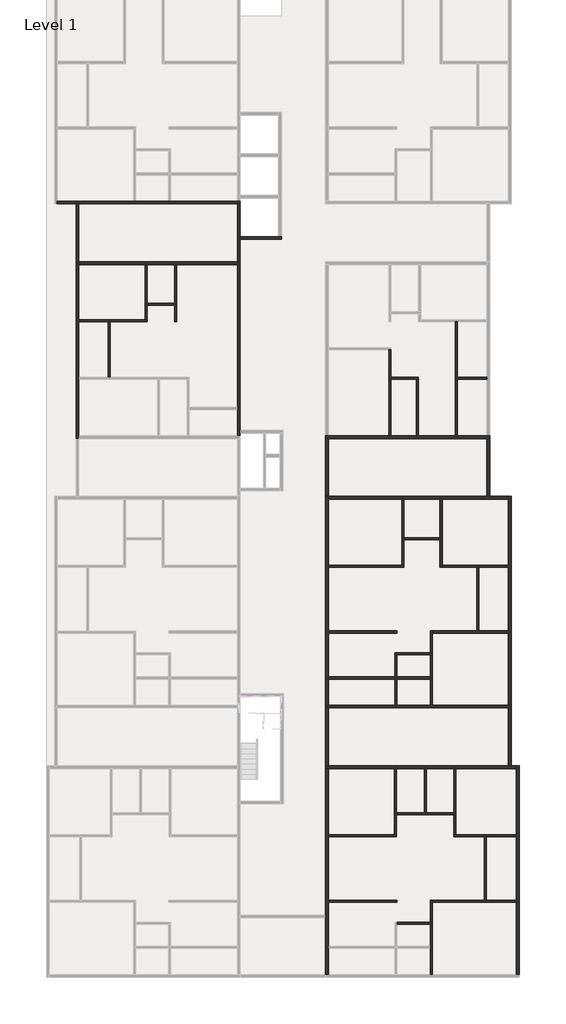
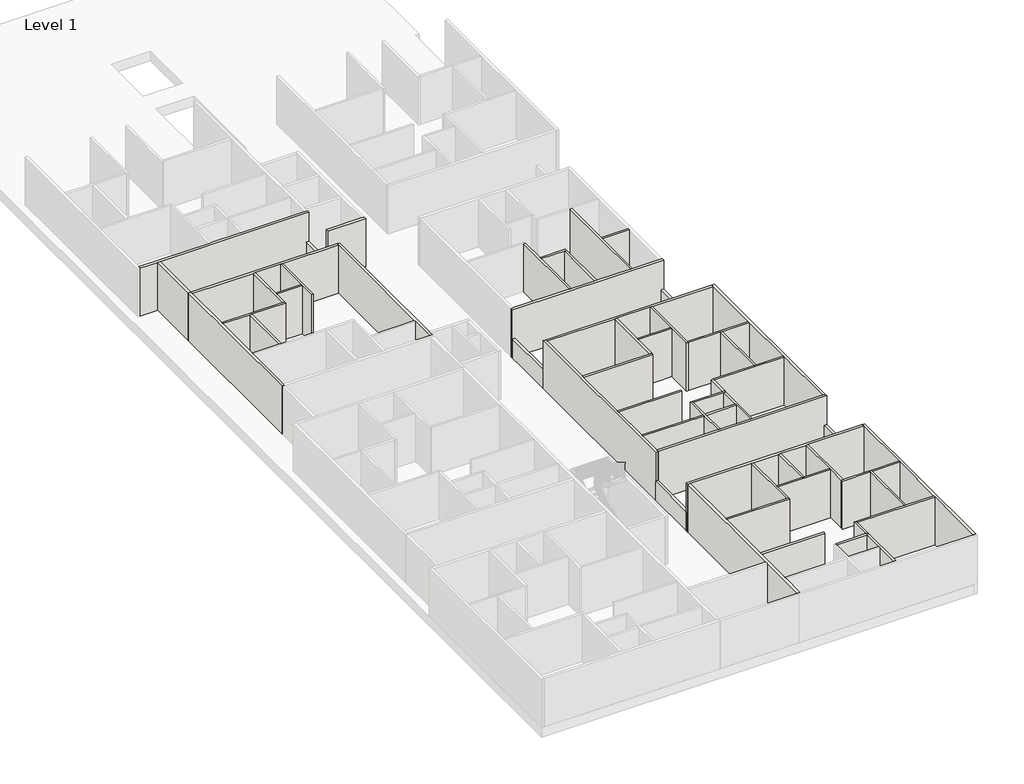
# One storey, part 2 of 8: 56 walls.
"""IFC4 building model written with IfcOpenShell, lengths in millimetres."""

from ifc_helpers import new_model, si_unit, frame, origin, place, context, project, spatial, polyline, outline, extrude, faceted_brep, element, save

model = new_model("IFC4")

# Units and contexts
model_context = context("Model", 3, world=origin())
ifc_project = project(units=[si_unit("LENGTHUNIT", "METRE", prefix="MILLI")], contexts=[model_context])

# Site, building, storey
site = spatial("IfcSite", under=ifc_project)
building = spatial("IfcBuilding", under=site)
storey = spatial("IfcBuildingStorey", under=building, Name="Level 1", Elevation=25234.6172466)

# Walls
placement = place(None, origin())
element("IfcWall", 1, ObjectType="4.5\"", at=placement, inside=storey, context=model_context, shape_type="Brep", body=[
    faceted_brep([(-12531.5544854, 2100.0216096, 25234.6172466), (-10907.2415084, 2100.0216096, 25234.6172466), (-10792.9415084, 2100.0216096, 25234.6172466), (-8759.6544854, 2100.0216096, 25234.6172466), (-8759.6544854, 2100.0216096, 28282.6172466), (-10792.9415084, 2100.0216096, 28282.6172466), (-10907.2415084, 2100.0216096, 28282.6172466), (-12531.5544854, 2100.0216096, 28282.6172466), (-12531.5544854, 2214.3216096, 25234.6172466), (-12531.5544854, 2214.3216096, 28282.6172466), (-8873.9544854, 2214.3216096, 28282.6172466), (-8759.6544854, 2214.3216096, 28282.6172466), (-8759.6544854, 2214.3216096, 25234.6172466), (-8873.9544854, 2214.3216096, 25234.6172466)], [[[0, 1, 2, 3, 4, 5, 6, 7]], [[8, 9, 10, 11, 12, 13]], [[3, 2, 1, 0, 8, 13, 12]], [[0, 7, 9, 8]], [[4, 3, 12, 11]], [[7, 6, 5, 4, 11, 10, 9]]]),
])
element("IfcWall", 2, ObjectType="4.5\"", at=placement, inside=storey, context=model_context, shape_type="Brep", body=[
    faceted_brep([(-8759.6544854, 2214.3216096, 25234.6172466), (-8759.6544854, 3014.4216096, 25234.6172466), (-8759.6544854, 3128.7216096, 25234.6172466), (-8759.6544854, 5264.2743917, 25234.6172466), (-8759.6544854, 5264.2743917, 28282.6172466), (-8759.6544854, 3128.7216096, 28282.6172466), (-8759.6544854, 3014.4216096, 28282.6172466), (-8759.6544854, 2214.3216096, 28282.6172466), (-8873.9544854, 2214.3216096, 25234.6172466), (-8873.9544854, 2214.3216096, 28282.6172466), (-8873.9544854, 5264.2743917, 28282.6172466), (-8873.9544854, 5264.2743917, 25234.6172466)], [[[0, 1, 2, 3, 4, 5, 6, 7]], [[8, 9, 10, 11]], [[3, 2, 1, 0, 8, 11]], [[0, 7, 9, 8]], [[4, 3, 11, 10]], [[7, 6, 5, 4, 10, 9]]]),
])
element("IfcWall", 3, ObjectType="4.5\"", at=placement, inside=storey, context=model_context, shape_type="Brep", body=[
    faceted_brep([(-7235.6544854, 5264.2743917, 25234.6172466), (-7235.6544854, 3128.7216096, 25234.6172466), (-7235.6544854, 3014.4216096, 25234.6172466), (-7235.6544854, 2100.0216096, 25234.6172466), (-7235.6544854, 2100.0216096, 28282.6172466), (-7235.6544854, 3014.4216096, 28282.6172466), (-7235.6544854, 3128.7216096, 28282.6172466), (-7235.6544854, 5264.2743917, 28282.6172466), (-7121.3544854, 5264.2743917, 25234.6172466), (-7121.3544854, 5264.2743917, 28282.6172466), (-7121.3544854, 2100.0216096, 28282.6172466), (-7121.3544854, 2100.0216096, 25234.6172466)], [[[0, 1, 2, 3, 4, 5, 6, 7]], [[8, 9, 10, 11]], [[3, 2, 1, 0, 8, 11]], [[4, 3, 11, 10]], [[0, 7, 9, 8]], [[7, 6, 5, 4, 10, 9]]]),
])
element("IfcWall", 4, ObjectType="4.5\"", at=placement, inside=storey, context=model_context, shape_type="SweptSolid", body=[
    extrude(outline(polyline([(-7235.6544854, 3014.4216096), (-8759.6544854, 3014.4216096), (-8759.6544854, 3128.7216096), (-7235.6544854, 3128.7216096), (-7235.6544854, 3014.4216096)])), frame((0.0, 0.0, 25234.6172466), z_axis=(0.0, 0.0, 1.0), x_axis=(1.0, 0.0, 0.0)), (0.0, 0.0, 1.0), 3048.0),
])
element("IfcWall", 5, ObjectType="4.5\"", at=placement, inside=storey, context=model_context, shape_type="SweptSolid", body=[
    extrude(outline(polyline([(-10907.2415084, -947.4344126), (-10907.2415084, 2100.0216096), (-10792.9415084, 2100.0216096), (-10792.9415084, -947.4344126), (-10907.2415084, -947.4344126)])), frame((0.0, 0.0, 25234.6172466), z_axis=(0.0, 0.0, 1.0), x_axis=(1.0, 0.0, 0.0)), (0.0, 0.0, 1.0), 3048.0),
])
element("IfcWall", 6, ObjectType="4.5\"", at=placement, inside=storey, context=model_context, shape_type="Brep", body=[
    faceted_brep([(5056.6584916, -31173.4344126, 25234.6172466), (6885.4584916, -31173.4344126, 25234.6172466), (6999.7584916, -31173.4344126, 25234.6172466), (6999.7584916, -31173.4344126, 28282.6172466), (6885.4584916, -31173.4344126, 28282.6172466), (5056.6584916, -31173.4344126, 28282.6172466), (5056.6584916, -31059.1344126, 25234.6172466), (5056.6584916, -31059.1344126, 28282.6172466), (6885.4584916, -31059.1344126, 28282.6172466), (6999.7584916, -31059.1344126, 28282.6172466), (6999.7584916, -31059.1344126, 25234.6172466), (6885.4584916, -31059.1344126, 25234.6172466)], [[[0, 1, 2, 3, 4, 5]], [[6, 7, 8, 9, 10, 11]], [[2, 1, 0, 6, 11, 10]], [[0, 5, 7, 6]], [[3, 2, 10, 9]], [[5, 4, 3, 9, 8, 7]]]),
])
element("IfcWall", 7, ObjectType="4.5\"", at=placement, inside=storey, context=model_context, shape_type="Brep", body=[
    faceted_brep([(6885.4584916, -31173.4344126, 25234.6172466), (6885.4584916, -32392.6344126, 25234.6172466), (6885.4584916, -32506.9344126, 25234.6172466), (6885.4584916, -33954.7344126, 25234.6172466), (6885.4584916, -33954.7344126, 28282.6172466), (6885.4584916, -32506.9344126, 28282.6172466), (6885.4584916, -32392.6344126, 28282.6172466), (6885.4584916, -31173.4344126, 28282.6172466), (6999.7584916, -31173.4344126, 25234.6172466), (6999.7584916, -31173.4344126, 28282.6172466), (6999.7584916, -33954.7344126, 28282.6172466), (6999.7584916, -33954.7344126, 25234.6172466)], [[[0, 1, 2, 3, 4, 5, 6, 7]], [[8, 9, 10, 11]], [[3, 2, 1, 0, 8, 11]], [[0, 7, 9, 8]], [[4, 3, 11, 10]], [[7, 6, 5, 4, 10, 9]]]),
])
element("IfcWall", 8, ObjectType="4.5\"", at=placement, inside=storey, context=model_context, shape_type="Brep", body=[
    faceted_brep([(6999.7584916, -31059.1344126, 25234.6172466), (6999.7584916, -29966.9344126, 25234.6172466), (6999.7584916, -29852.6344126, 25234.6172466), (6999.7584916, -29852.6344126, 28282.6172466), (6999.7584916, -29966.9344126, 28282.6172466), (6999.7584916, -31059.1344126, 28282.6172466), (6885.4584916, -31059.1344126, 25234.6172466), (6885.4584916, -31059.1344126, 28282.6172466), (6885.4584916, -29852.6344126, 28282.6172466), (6885.4584916, -29852.6344126, 25234.6172466)], [[[0, 1, 2, 3, 4, 5]], [[6, 7, 8, 9]], [[2, 1, 0, 6, 9]], [[0, 5, 7, 6]], [[3, 2, 9, 8]], [[5, 4, 3, 8, 7]]]),
])
element("IfcWall", 9, ObjectType="4.5\"", at=placement, inside=storey, context=model_context, shape_type="Brep", body=[
    faceted_brep([(6999.7584916, -29966.9344126, 25234.6172466), (11660.6584916, -29966.9344126, 25234.6172466), (11660.6584916, -29966.9344126, 28282.6172466), (6999.7584916, -29966.9344126, 28282.6172466), (6999.7584916, -29852.6344126, 25234.6172466), (6999.7584916, -29852.6344126, 28282.6172466), (9869.9584916, -29852.6344126, 28282.6172466), (9984.2584916, -29852.6344126, 28282.6172466), (11660.6584916, -29852.6344126, 28282.6172466), (11660.6584916, -29852.6344126, 25234.6172466), (9984.2584916, -29852.6344126, 25234.6172466), (9869.9584916, -29852.6344126, 25234.6172466)], [[[0, 1, 2, 3]], [[4, 5, 6, 7, 8, 9, 10, 11]], [[1, 0, 4, 11, 10, 9]], [[0, 3, 5, 4]], [[2, 1, 9, 8]], [[3, 2, 8, 7, 6, 5]]]),
])
element("IfcWall", 10, ObjectType="4.5\"", at=placement, inside=storey, context=model_context, shape_type="SweptSolid", body=[
    extrude(outline(polyline([(5056.6584916, -29966.9344126), (1259.3584916, -29966.9344126), (1259.3584916, -29852.6344126), (5056.6584916, -29852.6344126), (5056.6584916, -29966.9344126)])), frame((0.0, 0.0, 25234.6172466), z_axis=(0.0, 0.0, 1.0), x_axis=(1.0, 0.0, 0.0)), (0.0, 0.0, 1.0), 3048.0),
])
element("IfcWall", 11, ObjectType="4.5\"", at=placement, inside=storey, context=model_context, shape_type="Brep", body=[
    faceted_brep([(1259.3584916, -26347.4344126, 25234.6172466), (5031.2584916, -26347.4344126, 25234.6172466), (5031.2584916, -26347.4344126, 28282.6172466), (1259.3584916, -26347.4344126, 28282.6172466), (1259.3584916, -26233.1344126, 25234.6172466), (1259.3584916, -26233.1344126, 28282.6172466), (4916.9584916, -26233.1344126, 28282.6172466), (5031.2584916, -26233.1344126, 28282.6172466), (5031.2584916, -26233.1344126, 25234.6172466), (4916.9584916, -26233.1344126, 25234.6172466)], [[[0, 1, 2, 3]], [[4, 5, 6, 7, 8, 9]], [[1, 0, 4, 9, 8]], [[0, 3, 5, 4]], [[2, 1, 8, 7]], [[3, 2, 7, 6, 5]]]),
])
element("IfcWall", 12, ObjectType="4.5\"", at=placement, inside=storey, context=model_context, shape_type="Brep", body=[
    faceted_brep([(5031.2584916, -26233.1344126, 25234.6172466), (5031.2584916, -25128.2344126, 25234.6172466), (5031.2584916, -25013.9344126, 25234.6172466), (5031.2584916, -22575.5344126, 25234.6172466), (5031.2584916, -22575.5344126, 28282.6172466), (5031.2584916, -25013.9344126, 28282.6172466), (5031.2584916, -25128.2344126, 28282.6172466), (5031.2584916, -26233.1344126, 28282.6172466), (4916.9584916, -26233.1344126, 25234.6172466), (4916.9584916, -26233.1344126, 28282.6172466), (4916.9584916, -22575.5344126, 28282.6172466), (4916.9584916, -22575.5344126, 25234.6172466)], [[[0, 1, 2, 3, 4, 5, 6, 7]], [[8, 9, 10, 11]], [[3, 2, 1, 0, 8, 11]], [[0, 7, 9, 8]], [[4, 3, 11, 10]], [[7, 6, 5, 4, 10, 9]]]),
])
element("IfcWall", 13, ObjectType="4.5\"", at=placement, inside=storey, context=model_context, shape_type="Brep", body=[
    faceted_brep([(9984.2584916, -29852.6344126, 25234.6172466), (9984.2584916, -26347.4344126, 25234.6172466), (9984.2584916, -26233.1344126, 25234.6172466), (9984.2584916, -26233.1344126, 28282.6172466), (9984.2584916, -26347.4344126, 28282.6172466), (9984.2584916, -29852.6344126, 28282.6172466), (9869.9584916, -29852.6344126, 25234.6172466), (9869.9584916, -29852.6344126, 28282.6172466), (9869.9584916, -26347.4344126, 28282.6172466), (9869.9584916, -26233.1344126, 28282.6172466), (9869.9584916, -26233.1344126, 25234.6172466), (9869.9584916, -26347.4344126, 25234.6172466)], [[[0, 1, 2, 3, 4, 5]], [[6, 7, 8, 9, 10, 11]], [[2, 1, 0, 6, 11, 10]], [[0, 5, 7, 6]], [[3, 2, 10, 9]], [[5, 4, 3, 9, 8, 7]]]),
])
element("IfcWall", 14, ObjectType="4.5\"", at=placement, inside=storey, context=model_context, shape_type="SweptSolid", body=[
    extrude(outline(polyline([(11660.6584916, -26347.4344126), (9984.2584916, -26347.4344126), (9984.2584916, -26233.1344126), (11660.6584916, -26233.1344126), (11660.6584916, -26347.4344126)])), frame((0.0, 0.0, 25234.6172466), z_axis=(0.0, 0.0, 1.0), x_axis=(1.0, 0.0, 0.0)), (0.0, 0.0, 1.0), 3048.0),
])
element("IfcWall", 15, ObjectType="4.5\"", at=placement, inside=storey, context=model_context, shape_type="Brep", body=[
    faceted_brep([(9869.9584916, -26233.1344126, 25234.6172466), (8307.8584916, -26233.1344126, 25234.6172466), (8193.5584916, -26233.1344126, 25234.6172466), (8193.5584916, -26233.1344126, 28282.6172466), (8307.8584916, -26233.1344126, 28282.6172466), (9869.9584916, -26233.1344126, 28282.6172466), (9869.9584916, -26347.4344126, 25234.6172466), (9869.9584916, -26347.4344126, 28282.6172466), (8193.5584916, -26347.4344126, 28282.6172466), (8193.5584916, -26347.4344126, 25234.6172466)], [[[0, 1, 2, 3, 4, 5]], [[6, 7, 8, 9]], [[2, 1, 0, 6, 9]], [[0, 5, 7, 6]], [[3, 2, 9, 8]], [[5, 4, 3, 8, 7]]]),
])
element("IfcWall", 16, ObjectType="4.5\"", at=placement, inside=storey, context=model_context, shape_type="Brep", body=[
    faceted_brep([(8307.8584916, -26233.1344126, 25234.6172466), (8307.8584916, -22575.5344126, 25234.6172466), (8307.8584916, -22575.5344126, 28282.6172466), (8307.8584916, -26233.1344126, 28282.6172466), (8193.5584916, -26233.1344126, 25234.6172466), (8193.5584916, -26233.1344126, 28282.6172466), (8193.5584916, -25128.2344126, 28282.6172466), (8193.5584916, -25013.9344126, 28282.6172466), (8193.5584916, -22575.5344126, 28282.6172466), (8193.5584916, -22575.5344126, 25234.6172466), (8193.5584916, -25013.9344126, 25234.6172466), (8193.5584916, -25128.2344126, 25234.6172466)], [[[0, 1, 2, 3]], [[4, 5, 6, 7, 8, 9, 10, 11]], [[1, 0, 4, 11, 10, 9]], [[0, 3, 5, 4]], [[2, 1, 9, 8]], [[3, 2, 8, 7, 6, 5]]]),
])
element("IfcWall", 17, ObjectType="4.5\"", at=placement, inside=storey, context=model_context, shape_type="Brep", body=[
    faceted_brep([(5031.2584916, -25128.2344126, 25234.6172466), (8193.5584916, -25128.2344126, 25234.6172466), (8193.5584916, -25128.2344126, 28282.6172466), (5031.2584916, -25128.2344126, 28282.6172466), (5031.2584916, -25013.9344126, 25234.6172466), (5031.2584916, -25013.9344126, 28282.6172466), (6555.2584916, -25013.9344126, 28282.6172466), (6669.5584916, -25013.9344126, 28282.6172466), (8193.5584916, -25013.9344126, 28282.6172466), (8193.5584916, -25013.9344126, 25234.6172466), (6669.5584916, -25013.9344126, 25234.6172466), (6555.2584916, -25013.9344126, 25234.6172466)], [[[0, 1, 2, 3]], [[4, 5, 6, 7, 8, 9, 10, 11]], [[1, 0, 4, 11, 10, 9]], [[0, 3, 5, 4]], [[2, 1, 9, 8]], [[3, 2, 8, 7, 6, 5]]]),
])
element("IfcWall", 18, ObjectType="4.5\"", at=placement, inside=storey, context=model_context, shape_type="SweptSolid", body=[
    extrude(outline(polyline([(6555.2584916, -25013.9344126), (6555.2584916, -22575.5344126), (6669.5584916, -22575.5344126), (6669.5584916, -25013.9344126), (6555.2584916, -25013.9344126)])), frame((0.0, 0.0, 25234.6172466), z_axis=(0.0, 0.0, 1.0), x_axis=(1.0, 0.0, 0.0)), (0.0, 0.0, 1.0), 3048.0),
])
element("IfcWall", 19, ObjectType="4.5\"", at=placement, inside=storey, context=model_context, shape_type="SweptSolid", body=[
    extrude(outline(polyline([(4942.3584916, -17622.5344126), (1259.3584916, -17622.5344126), (1259.3584916, -17508.2344126), (4942.3584916, -17508.2344126), (4942.3584916, -17622.5344126)])), frame((0.0, 0.0, 25234.6172466), z_axis=(0.0, 0.0, 1.0), x_axis=(1.0, 0.0, 0.0)), (0.0, 0.0, 1.0), 3048.0),
])
element("IfcWall", 20, ObjectType="4.5\"", at=placement, inside=storey, context=model_context, shape_type="Brep", body=[
    faceted_brep([(4942.3584916, -16174.7344126, 25234.6172466), (4942.3584916, -17508.2344126, 25234.6172466), (4942.3584916, -17622.5344126, 25234.6172466), (4942.3584916, -19070.3344126, 25234.6172466), (4942.3584916, -19070.3344126, 28282.6172466), (4942.3584916, -17622.5344126, 28282.6172466), (4942.3584916, -17508.2344126, 28282.6172466), (4942.3584916, -16174.7344126, 28282.6172466), (5056.6584916, -16174.7344126, 25234.6172466), (5056.6584916, -16174.7344126, 28282.6172466), (5056.6584916, -16289.0344126, 28282.6172466), (5056.6584916, -17508.2344126, 28282.6172466), (5056.6584916, -17622.5344126, 28282.6172466), (5056.6584916, -19070.3344126, 28282.6172466), (5056.6584916, -19070.3344126, 25234.6172466), (5056.6584916, -17622.5344126, 25234.6172466), (5056.6584916, -17508.2344126, 25234.6172466), (5056.6584916, -16289.0344126, 25234.6172466)], [[[0, 1, 2, 3, 4, 5, 6, 7]], [[8, 9, 10, 11, 12, 13, 14, 15, 16, 17]], [[3, 2, 1, 0, 8, 17, 16, 15, 14]], [[4, 3, 14, 13]], [[0, 7, 9, 8]], [[7, 6, 5, 4, 13, 12, 11, 10, 9]]]),
])
element("IfcWall", 21, ObjectType="4.5\"", at=placement, inside=storey, context=model_context, shape_type="Brep", body=[
    faceted_brep([(5056.6584916, -16289.0344126, 25234.6172466), (6885.4584916, -16289.0344126, 25234.6172466), (6999.7584916, -16289.0344126, 25234.6172466), (6999.7584916, -16289.0344126, 28282.6172466), (6885.4584916, -16289.0344126, 28282.6172466), (5056.6584916, -16289.0344126, 28282.6172466), (5056.6584916, -16174.7344126, 25234.6172466), (5056.6584916, -16174.7344126, 28282.6172466), (6885.4584916, -16174.7344126, 28282.6172466), (6999.7584916, -16174.7344126, 28282.6172466), (6999.7584916, -16174.7344126, 25234.6172466), (6885.4584916, -16174.7344126, 25234.6172466)], [[[0, 1, 2, 3, 4, 5]], [[6, 7, 8, 9, 10, 11]], [[2, 1, 0, 6, 11, 10]], [[0, 5, 7, 6]], [[3, 2, 10, 9]], [[5, 4, 3, 9, 8, 7]]]),
])
element("IfcWall", 22, ObjectType="4.5\"", at=placement, inside=storey, context=model_context, shape_type="Brep", body=[
    faceted_brep([(6885.4584916, -16289.0344126, 25234.6172466), (6885.4584916, -17508.2344126, 25234.6172466), (6885.4584916, -17622.5344126, 25234.6172466), (6885.4584916, -19070.3344126, 25234.6172466), (6885.4584916, -19070.3344126, 28282.6172466), (6885.4584916, -17622.5344126, 28282.6172466), (6885.4584916, -17508.2344126, 28282.6172466), (6885.4584916, -16289.0344126, 28282.6172466), (6999.7584916, -16289.0344126, 25234.6172466), (6999.7584916, -16289.0344126, 28282.6172466), (6999.7584916, -19070.3344126, 28282.6172466), (6999.7584916, -19070.3344126, 25234.6172466)], [[[0, 1, 2, 3, 4, 5, 6, 7]], [[8, 9, 10, 11]], [[3, 2, 1, 0, 8, 11]], [[0, 7, 9, 8]], [[4, 3, 11, 10]], [[7, 6, 5, 4, 10, 9]]]),
])
element("IfcWall", 23, ObjectType="4.5\"", at=placement, inside=storey, context=model_context, shape_type="SweptSolid", body=[
    extrude(outline(polyline([(6885.4584916, -17622.5344126), (5056.6584916, -17622.5344126), (5056.6584916, -17508.2344126), (6885.4584916, -17508.2344126), (6885.4584916, -17622.5344126)])), frame((0.0, 0.0, 25234.6172466), z_axis=(0.0, 0.0, 1.0), x_axis=(1.0, 0.0, 0.0)), (0.0, 0.0, 1.0), 3048.0),
])
element("IfcWall", 24, ObjectType="4.5\"", at=placement, inside=storey, context=model_context, shape_type="Brep", body=[
    faceted_brep([(6999.7584916, -16174.7344126, 25234.6172466), (6999.7584916, -15082.5344126, 25234.6172466), (6999.7584916, -14968.2344126, 25234.6172466), (6999.7584916, -14968.2344126, 28282.6172466), (6999.7584916, -15082.5344126, 28282.6172466), (6999.7584916, -16174.7344126, 28282.6172466), (6885.4584916, -16174.7344126, 25234.6172466), (6885.4584916, -16174.7344126, 28282.6172466), (6885.4584916, -14968.2344126, 28282.6172466), (6885.4584916, -14968.2344126, 25234.6172466)], [[[0, 1, 2, 3, 4, 5]], [[6, 7, 8, 9]], [[2, 1, 0, 6, 9]], [[0, 5, 7, 6]], [[3, 2, 9, 8]], [[5, 4, 3, 8, 7]]]),
])
element("IfcWall", 25, ObjectType="4.5\"", at=placement, inside=storey, context=model_context, shape_type="Brep", body=[
    faceted_brep([(6999.7584916, -15082.5344126, 25234.6172466), (11208.5214687, -15082.5344126, 25234.6172466), (11208.5214687, -15082.5344126, 28282.6172466), (6999.7584916, -15082.5344126, 28282.6172466), (6999.7584916, -14968.2344126, 25234.6172466), (6999.7584916, -14968.2344126, 28282.6172466), (9469.9084916, -14968.2344126, 28282.6172466), (9584.2084916, -14968.2344126, 28282.6172466), (11208.5214687, -14968.2344126, 28282.6172466), (11208.5214687, -14968.2344126, 25234.6172466), (9584.2084916, -14968.2344126, 25234.6172466), (9469.9084916, -14968.2344126, 25234.6172466)], [[[0, 1, 2, 3]], [[4, 5, 6, 7, 8, 9, 10, 11]], [[1, 0, 4, 11, 10, 9]], [[0, 3, 5, 4]], [[2, 1, 9, 8]], [[3, 2, 8, 7, 6, 5]]]),
])
element("IfcWall", 26, ObjectType="4.5\"", at=placement, inside=storey, context=model_context, shape_type="SweptSolid", body=[
    extrude(outline(polyline([(5056.6584916, -15082.5344126), (1259.3584916, -15082.5344126), (1259.3584916, -14968.2344126), (5056.6584916, -14968.2344126), (5056.6584916, -15082.5344126)])), frame((0.0, 0.0, 25234.6172466), z_axis=(0.0, 0.0, 1.0), x_axis=(1.0, 0.0, 0.0)), (0.0, 0.0, 1.0), 3048.0),
])
element("IfcWall", 27, ObjectType="4.5\"", at=placement, inside=storey, context=model_context, shape_type="Brep", body=[
    faceted_brep([(1259.3584916, -11463.0344126, 25234.6172466), (5430.0214687, -11463.0344126, 25234.6172466), (5430.0214687, -11463.0344126, 28282.6172466), (1259.3584916, -11463.0344126, 28282.6172466), (1259.3584916, -11348.7344126, 25234.6172466), (1259.3584916, -11348.7344126, 28282.6172466), (5315.7214687, -11348.7344126, 28282.6172466), (5430.0214687, -11348.7344126, 28282.6172466), (5430.0214687, -11348.7344126, 25234.6172466), (5315.7214687, -11348.7344126, 25234.6172466)], [[[0, 1, 2, 3]], [[4, 5, 6, 7, 8, 9]], [[1, 0, 4, 9, 8]], [[0, 3, 5, 4]], [[2, 1, 8, 7]], [[3, 2, 7, 6, 5]]]),
])
element("IfcWall", 28, ObjectType="4.5\"", at=placement, inside=storey, context=model_context, shape_type="Brep", body=[
    faceted_brep([(5430.0214687, -11348.7344126, 25234.6172466), (5430.0214687, -9939.0344126, 25234.6172466), (5430.0214687, -9824.7344126, 25234.6172466), (5430.0214687, -7691.1344126, 25234.6172466), (5430.0214687, -7691.1344126, 28282.6172466), (5430.0214687, -9824.7344126, 28282.6172466), (5430.0214687, -9939.0344126, 28282.6172466), (5430.0214687, -11348.7344126, 28282.6172466), (5315.7214687, -11348.7344126, 25234.6172466), (5315.7214687, -11348.7344126, 28282.6172466), (5315.7214687, -7691.1344126, 28282.6172466), (5315.7214687, -7691.1344126, 25234.6172466)], [[[0, 1, 2, 3, 4, 5, 6, 7]], [[8, 9, 10, 11]], [[3, 2, 1, 0, 8, 11]], [[0, 7, 9, 8]], [[4, 3, 11, 10]], [[7, 6, 5, 4, 10, 9]]]),
])
element("IfcWall", 29, ObjectType="4.5\"", at=placement, inside=storey, context=model_context, shape_type="SweptSolid", body=[
    extrude(outline(polyline([(7436.6214687, -9939.0344126), (5430.0214687, -9939.0344126), (5430.0214687, -9824.7344126), (7436.6214687, -9824.7344126), (7436.6214687, -9939.0344126)])), frame((0.0, 0.0, 25234.6172466), z_axis=(0.0, 0.0, 1.0), x_axis=(1.0, 0.0, 0.0)), (0.0, 0.0, 1.0), 3048.0),
])
element("IfcWall", 30, ObjectType="4.5\"", at=placement, inside=storey, context=model_context, shape_type="Brep", body=[
    faceted_brep([(7436.6214687, -7691.1344126, 25234.6172466), (7436.6214687, -9824.7344126, 25234.6172466), (7436.6214687, -9939.0344126, 25234.6172466), (7436.6214687, -11463.0344126, 25234.6172466), (7436.6214687, -11463.0344126, 28282.6172466), (7436.6214687, -9939.0344126, 28282.6172466), (7436.6214687, -9824.7344126, 28282.6172466), (7436.6214687, -7691.1344126, 28282.6172466), (7550.9214687, -7691.1344126, 25234.6172466), (7550.9214687, -7691.1344126, 28282.6172466), (7550.9214687, -11348.7344126, 28282.6172466), (7550.9214687, -11463.0344126, 28282.6172466), (7550.9214687, -11463.0344126, 25234.6172466), (7550.9214687, -11348.7344126, 25234.6172466)], [[[0, 1, 2, 3, 4, 5, 6, 7]], [[8, 9, 10, 11, 12, 13]], [[3, 2, 1, 0, 8, 13, 12]], [[0, 7, 9, 8]], [[4, 3, 12, 11]], [[7, 6, 5, 4, 11, 10, 9]]]),
])
element("IfcWall", 31, ObjectType="4.5\"", at=placement, inside=storey, context=model_context, shape_type="Brep", body=[
    faceted_brep([(7550.9214687, -11463.0344126, 25234.6172466), (9469.9084916, -11463.0344126, 25234.6172466), (9584.2084916, -11463.0344126, 25234.6172466), (11208.5214687, -11463.0344126, 25234.6172466), (11208.5214687, -11463.0344126, 28282.6172466), (9584.2084916, -11463.0344126, 28282.6172466), (9469.9084916, -11463.0344126, 28282.6172466), (7550.9214687, -11463.0344126, 28282.6172466), (7550.9214687, -11348.7344126, 25234.6172466), (7550.9214687, -11348.7344126, 28282.6172466), (11208.5214687, -11348.7344126, 28282.6172466), (11208.5214687, -11348.7344126, 25234.6172466)], [[[0, 1, 2, 3, 4, 5, 6, 7]], [[8, 9, 10, 11]], [[3, 2, 1, 0, 8, 11]], [[0, 7, 9, 8]], [[4, 3, 11, 10]], [[7, 6, 5, 4, 10, 9]]]),
])
element("IfcWall", 32, ObjectType="4.5\"", at=placement, inside=storey, context=model_context, shape_type="SweptSolid", body=[
    extrude(outline(polyline([(9469.9084916, -14968.2344126), (9469.9084916, -11463.0344126), (9584.2084916, -11463.0344126), (9584.2084916, -14968.2344126), (9469.9084916, -14968.2344126)])), frame((0.0, 0.0, 25234.6172466), z_axis=(0.0, 0.0, 1.0), x_axis=(1.0, 0.0, 0.0)), (0.0, 0.0, 1.0), 3048.0),
])
element("IfcWall", 33, ObjectType="4.5\"", at=placement, inside=storey, context=model_context, shape_type="Brep", body=[
    faceted_brep([(4610.8714687, 572.7745083, 25234.6172466), (4610.8714687, -4185.9344126, 25234.6172466), (4610.8714687, -4185.9344126, 28282.6172466), (4610.8714687, 572.7745083, 28282.6172466), (4725.1714687, 572.7745083, 25234.6172466), (4725.1714687, 572.7745083, 28282.6172466), (4725.1714687, -947.4344126, 28282.6172466), (4725.1714687, -1061.7344126, 28282.6172466), (4725.1714687, -4185.9344126, 28282.6172466), (4725.1714687, -4185.9344126, 25234.6172466), (4725.1714687, -1061.7344126, 25234.6172466), (4725.1714687, -947.4344126, 25234.6172466)], [[[0, 1, 2, 3]], [[4, 5, 6, 7, 8, 9, 10, 11]], [[1, 0, 4, 11, 10, 9]], [[0, 3, 5, 4]], [[2, 1, 9, 8]], [[3, 2, 8, 7, 6, 5]]]),
])
element("IfcWall", 34, ObjectType="4.5\"", at=placement, inside=storey, context=model_context, shape_type="Brep", body=[
    faceted_brep([(4725.1714687, -1061.7344126, 25234.6172466), (6134.8714687, -1061.7344126, 25234.6172466), (6249.1714687, -1061.7344126, 25234.6172466), (6249.1714687, -1061.7344126, 28282.6172466), (6134.8714687, -1061.7344126, 28282.6172466), (4725.1714687, -1061.7344126, 28282.6172466), (4725.1714687, -947.4344126, 25234.6172466), (4725.1714687, -947.4344126, 28282.6172466), (6249.1714687, -947.4344126, 28282.6172466), (6249.1714687, -947.4344126, 25234.6172466)], [[[0, 1, 2, 3, 4, 5]], [[6, 7, 8, 9]], [[2, 1, 0, 6, 9]], [[0, 5, 7, 6]], [[3, 2, 9, 8]], [[5, 4, 3, 8, 7]]]),
])
element("IfcWall", 35, ObjectType="4.5\"", at=placement, inside=storey, context=model_context, shape_type="SweptSolid", body=[
    extrude(outline(polyline([(6134.8714687, -4185.9344126), (6134.8714687, -1061.7344126), (6249.1714687, -1061.7344126), (6249.1714687, -4185.9344126), (6134.8714687, -4185.9344126)])), frame((0.0, 0.0, 25234.6172466), z_axis=(0.0, 0.0, 1.0), x_axis=(1.0, 0.0, 0.0)), (0.0, 0.0, 1.0), 3048.0),
])
element("IfcWall", 36, ObjectType="4.5\"", at=placement, inside=storey, context=model_context, shape_type="Brep", body=[
    faceted_brep([(8396.7584916, -4185.9344126, 25234.6172466), (8396.7584916, -1061.7344126, 25234.6172466), (8396.7584916, -947.4344126, 25234.6172466), (8396.7584916, 2100.0216096, 25234.6172466), (8396.7584916, 2100.0216096, 28282.6172466), (8396.7584916, -947.4344126, 28282.6172466), (8396.7584916, -1061.7344126, 28282.6172466), (8396.7584916, -4185.9344126, 28282.6172466), (8282.4584916, -4185.9344126, 25234.6172466), (8282.4584916, -4185.9344126, 28282.6172466), (8282.4584916, 2100.0216096, 28282.6172466), (8282.4584916, 2100.0216096, 25234.6172466)], [[[0, 1, 2, 3, 4, 5, 6, 7]], [[8, 9, 10, 11]], [[3, 2, 1, 0, 8, 11]], [[0, 7, 9, 8]], [[4, 3, 11, 10]], [[7, 6, 5, 4, 10, 9]]]),
])
element("IfcWall", 37, ObjectType="4.5\"", at=placement, inside=storey, context=model_context, shape_type="SweptSolid", body=[
    extrude(outline(polyline([(8396.7584916, -947.4344126), (10021.0714687, -947.4344126), (10021.0714687, -1061.7344126), (8396.7584916, -1061.7344126), (8396.7584916, -947.4344126)])), frame((0.0, 0.0, 25234.6172466), z_axis=(0.0, 0.0, 1.0), x_axis=(1.0, 0.0, 0.0)), (0.0, 0.0, 1.0), 3048.0),
])
element("IfcWall", 38, ObjectType="6\"", at=placement, inside=storey, context=model_context, shape_type="Brep", body=[
    faceted_brep([(-13719.0044854, 8615.1216096, 25234.6172466), (-12683.9544854, 8615.1216096, 25234.6172466), (-12531.5544854, 8615.1216096, 25234.6172466), (-3769.8415084, 8615.1216096, 25234.6172466), (-3617.4415084, 8615.1216096, 25234.6172466), (-3617.4415084, 8615.1216096, 26453.8172466), (-3617.4415084, 8615.1216096, 28282.6172466), (-12531.5544854, 8615.1216096, 28282.6172466), (-12683.9544854, 8615.1216096, 28282.6172466), (-13719.0044854, 8615.1216096, 28282.6172466), (-13719.0044854, 8767.5216096, 25234.6172466), (-13719.0044854, 8767.5216096, 28282.6172466), (-9510.2415084, 8767.5216096, 28282.6172466), (-9395.9415084, 8767.5216096, 28282.6172466), (-7567.1415084, 8767.5216096, 28282.6172466), (-7452.8415084, 8767.5216096, 28282.6172466), (-3769.8415084, 8767.5216096, 28282.6172466), (-3617.4415084, 8767.5216096, 28282.6172466), (-3617.4415084, 8767.5216096, 25234.6172466), (-3769.8415084, 8767.5216096, 25234.6172466), (-7452.8415084, 8767.5216096, 25234.6172466), (-7567.1415084, 8767.5216096, 25234.6172466), (-9395.9415084, 8767.5216096, 25234.6172466), (-9510.2415084, 8767.5216096, 25234.6172466)], [[[0, 1, 2, 3, 4, 5, 6, 7, 8, 9]], [[10, 11, 12, 13, 14, 15, 16, 17, 18, 19, 20, 21, 22, 23]], [[4, 3, 2, 1, 0, 10, 23, 22, 21, 20, 19, 18]], [[0, 9, 11, 10]], [[4, 18, 17, 6, 5]], [[9, 8, 7, 6, 17, 16, 15, 14, 13, 12, 11]]]),
])
element("IfcWall", 39, ObjectType="6\"", at=placement, inside=storey, context=model_context, shape_type="Brep", body=[
    faceted_brep([(-12683.9544854, 5416.6743917, 25234.6172466), (-12683.9544854, -4338.3344126, 25234.6172466), (-12683.9544854, -4338.3344126, 28282.6172466), (-12683.9544854, 5416.6743917, 28282.6172466), (-12531.5544854, 5416.6743917, 25234.6172466), (-12531.5544854, 5416.6743917, 28282.6172466), (-12531.5544854, 5264.2743917, 28282.6172466), (-12531.5544854, 2214.3216096, 28282.6172466), (-12531.5544854, 2100.0216096, 28282.6172466), (-12531.5544854, -947.4344126, 28282.6172466), (-12531.5544854, -1061.7344126, 28282.6172466), (-12531.5544854, -4185.9344126, 28282.6172466), (-12531.5544854, -4338.3344126, 28282.6172466), (-12531.5544854, -4338.3344126, 25234.6172466), (-12531.5544854, -4185.9344126, 25234.6172466), (-12531.5544854, -1061.7344126, 25234.6172466), (-12531.5544854, -947.4344126, 25234.6172466), (-12531.5544854, 2100.0216096, 25234.6172466), (-12531.5544854, 2214.3216096, 25234.6172466), (-12531.5544854, 5264.2743917, 25234.6172466)], [[[0, 1, 2, 3]], [[4, 5, 6, 7, 8, 9, 10, 11, 12, 13, 14, 15, 16, 17, 18, 19]], [[1, 0, 4, 19, 18, 17, 16, 15, 14, 13]], [[2, 1, 13, 12]], [[0, 3, 5, 4]], [[3, 2, 12, 11, 10, 9, 8, 7, 6, 5]]]),
])
element("IfcWall", 40, ObjectType="6\"", at=placement, inside=storey, context=model_context, shape_type="Brep", body=[
    faceted_brep([(-3617.4415084, -4185.9344126, 25234.6172466), (-3617.4415084, -4034.6751812, 25234.6172466), (-3617.4415084, -3882.2751812, 25234.6172466), (-3617.4415084, 5416.6743917, 25234.6172466), (-3617.4415084, 5416.6743917, 28282.6172466), (-3617.4415084, -3882.2751812, 28282.6172466), (-3617.4415084, -4034.6751812, 28282.6172466), (-3617.4415084, -4185.9344126, 28282.6172466), (-3769.8415084, -4185.9344126, 25234.6172466), (-3769.8415084, -4185.9344126, 28282.6172466), (-3769.8415084, -2738.1344126, 28282.6172466), (-3769.8415084, -2623.8344126, 28282.6172466), (-3769.8415084, 5264.2743917, 28282.6172466), (-3769.8415084, 5416.6743917, 28282.6172466), (-3769.8415084, 5416.6743917, 25234.6172466), (-3769.8415084, 5264.2743917, 25234.6172466), (-3769.8415084, -2623.8344126, 25234.6172466), (-3769.8415084, -2738.1344126, 25234.6172466)], [[[0, 1, 2, 3, 4, 5, 6, 7]], [[8, 9, 10, 11, 12, 13, 14, 15, 16, 17]], [[3, 2, 1, 0, 8, 17, 16, 15, 14]], [[0, 7, 9, 8]], [[3, 14, 13, 4]], [[7, 6, 5, 4, 13, 12, 11, 10, 9]]]),
])
element("IfcWall", 41, ObjectType="6\"", at=placement, inside=storey, context=model_context, shape_type="Brep", body=[
    faceted_brep([(-3769.8415084, 5416.6743917, 28282.6172466), (-3769.8415084, 5416.6743917, 25234.6172466), (-12531.5544854, 5416.6743917, 25234.6172466), (-12531.5544854, 5416.6743917, 28282.6172466), (-3769.8415084, 5264.2743917, 25234.6172466), (-3769.8415084, 5264.2743917, 28282.6172466), (-7121.3544854, 5264.2743917, 28282.6172466), (-7235.6544854, 5264.2743917, 28282.6172466), (-8759.6544854, 5264.2743917, 28282.6172466), (-8873.9544854, 5264.2743917, 28282.6172466), (-12531.5544854, 5264.2743917, 28282.6172466), (-12531.5544854, 5264.2743917, 25234.6172466), (-8873.9544854, 5264.2743917, 25234.6172466), (-8759.6544854, 5264.2743917, 25234.6172466), (-7235.6544854, 5264.2743917, 25234.6172466), (-7121.3544854, 5264.2743917, 25234.6172466)], [[[0, 1, 2, 3]], [[4, 5, 6, 7, 8, 9, 10, 11, 12, 13, 14, 15]], [[2, 1, 4, 15, 14, 13, 12, 11]], [[3, 2, 11, 10]], [[0, 5, 4, 1]], [[0, 3, 10, 9, 8, 7, 6, 5]]]),
])
element("IfcWall", 42, ObjectType="6\"", at=placement, inside=storey, context=model_context, shape_type="Brep", body=[
    faceted_brep([(11813.0584916, -33954.7344126, 25234.6172466), (11813.0584916, -22423.1344126, 25234.6172466), (11813.0584916, -22423.1344126, 28282.6172466), (11813.0584916, -33954.7344126, 28282.6172466), (11660.6584916, -33954.7344126, 25234.6172466), (11660.6584916, -33954.7344126, 28282.6172466), (11660.6584916, -29966.9344126, 28282.6172466), (11660.6584916, -29852.6344126, 28282.6172466), (11660.6584916, -26347.4344126, 28282.6172466), (11660.6584916, -26233.1344126, 28282.6172466), (11660.6584916, -22575.5344126, 28282.6172466), (11660.6584916, -22423.1344126, 28282.6172466), (11660.6584916, -22423.1344126, 25234.6172466), (11660.6584916, -22575.5344126, 25234.6172466), (11660.6584916, -26233.1344126, 25234.6172466), (11660.6584916, -26347.4344126, 25234.6172466), (11660.6584916, -29852.6344126, 25234.6172466), (11660.6584916, -29966.9344126, 25234.6172466)], [[[0, 1, 2, 3]], [[4, 5, 6, 7, 8, 9, 10, 11, 12, 13, 14, 15, 16, 17]], [[1, 0, 4, 17, 16, 15, 14, 13, 12]], [[0, 3, 5, 4]], [[2, 1, 12, 11]], [[3, 2, 11, 10, 9, 8, 7, 6, 5]]]),
])
element("IfcWall", 43, ObjectType="6\"", at=placement, inside=storey, context=model_context, shape_type="Brep", body=[
    faceted_brep([(11660.6584916, -22423.1344126, 25234.6172466), (11360.9214687, -22423.1344126, 25234.6172466), (11208.5214687, -22423.1344126, 25234.6172466), (1259.3584916, -22423.1344126, 25234.6172466), (1106.9584916, -22423.1344126, 25234.6172466), (1106.9584916, -22423.1344126, 26453.8172466), (1106.9584916, -22423.1344126, 28282.6172466), (11660.6584916, -22423.1344126, 28282.6172466), (11660.6584916, -22575.5344126, 25234.6172466), (11660.6584916, -22575.5344126, 28282.6172466), (8307.8584916, -22575.5344126, 28282.6172466), (8193.5584916, -22575.5344126, 28282.6172466), (6669.5584916, -22575.5344126, 28282.6172466), (6555.2584916, -22575.5344126, 28282.6172466), (5031.2584916, -22575.5344126, 28282.6172466), (4916.9584916, -22575.5344126, 28282.6172466), (1259.3584916, -22575.5344126, 28282.6172466), (1106.9584916, -22575.5344126, 28282.6172466), (1106.9584916, -22575.5344126, 25234.6172466), (1259.3584916, -22575.5344126, 25234.6172466), (4916.9584916, -22575.5344126, 25234.6172466), (5031.2584916, -22575.5344126, 25234.6172466), (6555.2584916, -22575.5344126, 25234.6172466), (6669.5584916, -22575.5344126, 25234.6172466), (8193.5584916, -22575.5344126, 25234.6172466), (8307.8584916, -22575.5344126, 25234.6172466)], [[[0, 1, 2, 3, 4, 5, 6, 7]], [[8, 9, 10, 11, 12, 13, 14, 15, 16, 17, 18, 19, 20, 21, 22, 23, 24, 25]], [[4, 3, 2, 1, 0, 8, 25, 24, 23, 22, 21, 20, 19, 18]], [[0, 7, 9, 8]], [[4, 18, 17, 6, 5]], [[7, 6, 17, 16, 15, 14, 13, 12, 11, 10, 9]]]),
])
element("IfcWall", 44, ObjectType="6\"", at=placement, inside=storey, context=model_context, shape_type="Brep", body=[
    faceted_brep([(1106.9584916, -22575.5344126, 28282.6172466), (1106.9584916, -22575.5344126, 25234.6172466), (1106.9584916, -30668.5325185, 25234.6172466), (1106.9584916, -30820.9325185, 25234.6172466), (1106.9584916, -33954.7344126, 25234.6172466), (1106.9584916, -33954.7344126, 28282.6172466), (1106.9584916, -30820.9325185, 28282.6172466), (1106.9584916, -30668.5325185, 28282.6172466), (1259.3584916, -22575.5344126, 25234.6172466), (1259.3584916, -22575.5344126, 28282.6172466), (1259.3584916, -26233.1344126, 28282.6172466), (1259.3584916, -26347.4344126, 28282.6172466), (1259.3584916, -29852.6344126, 28282.6172466), (1259.3584916, -29966.9344126, 28282.6172466), (1259.3584916, -32392.6344126, 28282.6172466), (1259.3584916, -32506.9344126, 28282.6172466), (1259.3584916, -33954.7344126, 28282.6172466), (1259.3584916, -33954.7344126, 25234.6172466), (1259.3584916, -32506.9344126, 25234.6172466), (1259.3584916, -32392.6344126, 25234.6172466), (1259.3584916, -29966.9344126, 25234.6172466), (1259.3584916, -29852.6344126, 25234.6172466), (1259.3584916, -26347.4344126, 25234.6172466), (1259.3584916, -26233.1344126, 25234.6172466)], [[[0, 1, 2, 3, 4, 5, 6, 7]], [[8, 9, 10, 11, 12, 13, 14, 15, 16, 17, 18, 19, 20, 21, 22, 23]], [[4, 3, 2, 1, 8, 23, 22, 21, 20, 19, 18, 17]], [[5, 4, 17, 16]], [[0, 9, 8, 1]], [[0, 7, 6, 5, 16, 15, 14, 13, 12, 11, 10, 9]]]),
])
element("IfcWall", 45, ObjectType="6\"", at=placement, inside=storey, context=model_context, shape_type="Brep", body=[
    faceted_brep([(1106.9584916, -7538.7344126, 28282.6172466), (1106.9584916, -7538.7344126, 25234.6172466), (1106.9584916, -19222.7344126, 25234.6172466), (1106.9584916, -19222.7344126, 28282.6172466), (1259.3584916, -7538.7344126, 25234.6172466), (1259.3584916, -7538.7344126, 28282.6172466), (1259.3584916, -7691.1344126, 28282.6172466), (1259.3584916, -11348.7344126, 28282.6172466), (1259.3584916, -11463.0344126, 28282.6172466), (1259.3584916, -14968.2344126, 28282.6172466), (1259.3584916, -15082.5344126, 28282.6172466), (1259.3584916, -17508.2344126, 28282.6172466), (1259.3584916, -17622.5344126, 28282.6172466), (1259.3584916, -19070.3344126, 28282.6172466), (1259.3584916, -19222.7344126, 28282.6172466), (1259.3584916, -19222.7344126, 25234.6172466), (1259.3584916, -19070.3344126, 25234.6172466), (1259.3584916, -17622.5344126, 25234.6172466), (1259.3584916, -17508.2344126, 25234.6172466), (1259.3584916, -15082.5344126, 25234.6172466), (1259.3584916, -14968.2344126, 25234.6172466), (1259.3584916, -11463.0344126, 25234.6172466), (1259.3584916, -11348.7344126, 25234.6172466), (1259.3584916, -7691.1344126, 25234.6172466)], [[[0, 1, 2, 3]], [[4, 5, 6, 7, 8, 9, 10, 11, 12, 13, 14, 15, 16, 17, 18, 19, 20, 21, 22, 23]], [[2, 1, 4, 23, 22, 21, 20, 19, 18, 17, 16, 15]], [[0, 5, 4, 1]], [[2, 15, 14, 3]], [[0, 3, 14, 13, 12, 11, 10, 9, 8, 7, 6, 5]]]),
])
element("IfcWall", 46, ObjectType="6\"", at=placement, inside=storey, context=model_context, shape_type="Brep", body=[
    faceted_brep([(1259.3584916, -19222.7344126, 28282.6172466), (1259.3584916, -19222.7344126, 25234.6172466), (11208.5214687, -19222.7344126, 25234.6172466), (11360.9214687, -19222.7344126, 25234.6172466), (11360.9214687, -19222.7344126, 26453.8172466), (11360.9214687, -19222.7344126, 28282.6172466), (1259.3584916, -19070.3344126, 25234.6172466), (1259.3584916, -19070.3344126, 28282.6172466), (4942.3584916, -19070.3344126, 28282.6172466), (5056.6584916, -19070.3344126, 28282.6172466), (6885.4584916, -19070.3344126, 28282.6172466), (6999.7584916, -19070.3344126, 28282.6172466), (11208.5214687, -19070.3344126, 28282.6172466), (11360.9214687, -19070.3344126, 28282.6172466), (11360.9214687, -19070.3344126, 25234.6172466), (11208.5214687, -19070.3344126, 25234.6172466), (6999.7584916, -19070.3344126, 25234.6172466), (6885.4584916, -19070.3344126, 25234.6172466), (5056.6584916, -19070.3344126, 25234.6172466), (4942.3584916, -19070.3344126, 25234.6172466)], [[[0, 1, 2, 3, 4, 5]], [[6, 7, 8, 9, 10, 11, 12, 13, 14, 15, 16, 17, 18, 19]], [[3, 2, 1, 6, 19, 18, 17, 16, 15, 14]], [[3, 14, 13, 5, 4]], [[0, 7, 6, 1]], [[0, 5, 13, 12, 11, 10, 9, 8, 7]]]),
])
element("IfcWall", 47, ObjectType="6\"", at=placement, inside=storey, context=model_context, shape_type="Brep", body=[
    faceted_brep([(11360.9214687, -19070.3344126, 28282.6172466), (11360.9214687, -19070.3344126, 25234.6172466), (11360.9214687, -7538.7344126, 25234.6172466), (11360.9214687, -7538.7344126, 28282.6172466), (11208.5214687, -19070.3344126, 25234.6172466), (11208.5214687, -19070.3344126, 28282.6172466), (11208.5214687, -15082.5344126, 28282.6172466), (11208.5214687, -14968.2344126, 28282.6172466), (11208.5214687, -11463.0344126, 28282.6172466), (11208.5214687, -11348.7344126, 28282.6172466), (11208.5214687, -7691.1344126, 28282.6172466), (11208.5214687, -7538.7344126, 28282.6172466), (11208.5214687, -7538.7344126, 25234.6172466), (11208.5214687, -7691.1344126, 25234.6172466), (11208.5214687, -11348.7344126, 25234.6172466), (11208.5214687, -11463.0344126, 25234.6172466), (11208.5214687, -14968.2344126, 25234.6172466), (11208.5214687, -15082.5344126, 25234.6172466)], [[[0, 1, 2, 3]], [[4, 5, 6, 7, 8, 9, 10, 11, 12, 13, 14, 15, 16, 17]], [[2, 1, 4, 17, 16, 15, 14, 13, 12]], [[3, 2, 12, 11]], [[0, 5, 4, 1]], [[0, 3, 11, 10, 9, 8, 7, 6, 5]]]),
])
element("IfcWall", 48, ObjectType="6\"", at=placement, inside=storey, context=model_context, shape_type="Brep", body=[
    faceted_brep([(11208.5214687, -7538.7344126, 25234.6172466), (10173.4714687, -7538.7344126, 25234.6172466), (10021.0714687, -7538.7344126, 25234.6172466), (1259.3584916, -7538.7344126, 25234.6172466), (1259.3584916, -7538.7344126, 28282.6172466), (11208.5214687, -7538.7344126, 28282.6172466), (11208.5214687, -7691.1344126, 25234.6172466), (11208.5214687, -7691.1344126, 28282.6172466), (7550.9214687, -7691.1344126, 28282.6172466), (7436.6214687, -7691.1344126, 28282.6172466), (5430.0214687, -7691.1344126, 28282.6172466), (5315.7214687, -7691.1344126, 28282.6172466), (1259.3584916, -7691.1344126, 28282.6172466), (1259.3584916, -7691.1344126, 25234.6172466), (5315.7214687, -7691.1344126, 25234.6172466), (5430.0214687, -7691.1344126, 25234.6172466), (7436.6214687, -7691.1344126, 25234.6172466), (7550.9214687, -7691.1344126, 25234.6172466)], [[[0, 1, 2, 3, 4, 5]], [[6, 7, 8, 9, 10, 11, 12, 13, 14, 15, 16, 17]], [[3, 2, 1, 0, 6, 17, 16, 15, 14, 13]], [[0, 5, 7, 6]], [[3, 13, 12, 4]], [[5, 4, 12, 11, 10, 9, 8, 7]]]),
])
element("IfcWall", 49, ObjectType="6\"", at=placement, inside=storey, context=model_context, shape_type="Brep", body=[
    faceted_brep([(1106.9584916, -4338.3344126, 28282.6172466), (1106.9584916, -4338.3344126, 26453.8172466), (1106.9584916, -4338.3344126, 25234.6172466), (1259.3584916, -4338.3344126, 25234.6172466), (10021.0714687, -4338.3344126, 25234.6172466), (10173.4714687, -4338.3344126, 25234.6172466), (10173.4714687, -4338.3344126, 26453.8172466), (10173.4714687, -4338.3344126, 28282.6172466), (1106.9584916, -4185.9344126, 25234.6172466), (1106.9584916, -4185.9344126, 28282.6172466), (1259.3584916, -4185.9344126, 28282.6172466), (4610.8714687, -4185.9344126, 28282.6172466), (4725.1714687, -4185.9344126, 28282.6172466), (6134.8714687, -4185.9344126, 28282.6172466), (6249.1714687, -4185.9344126, 28282.6172466), (8282.4584916, -4185.9344126, 28282.6172466), (8396.7584916, -4185.9344126, 28282.6172466), (10021.0714687, -4185.9344126, 28282.6172466), (10173.4714687, -4185.9344126, 28282.6172466), (10173.4714687, -4185.9344126, 25234.6172466), (10021.0714687, -4185.9344126, 25234.6172466), (8396.7584916, -4185.9344126, 25234.6172466), (8282.4584916, -4185.9344126, 25234.6172466), (6249.1714687, -4185.9344126, 25234.6172466), (6134.8714687, -4185.9344126, 25234.6172466), (4725.1714687, -4185.9344126, 25234.6172466), (4610.8714687, -4185.9344126, 25234.6172466), (1259.3584916, -4185.9344126, 25234.6172466)], [[[0, 1, 2, 3, 4, 5, 6, 7]], [[8, 9, 10, 11, 12, 13, 14, 15, 16, 17, 18, 19, 20, 21, 22, 23, 24, 25, 26, 27]], [[5, 4, 3, 2, 8, 27, 26, 25, 24, 23, 22, 21, 20, 19]], [[0, 9, 8, 2, 1]], [[5, 19, 18, 7, 6]], [[0, 7, 18, 17, 16, 15, 14, 13, 12, 11, 10, 9]]]),
])
element("IfcWall", 50, ObjectType="6\"", at=placement, inside=storey, context=model_context, shape_type="Brep", body=[
    faceted_brep([(-3617.4415084, 6659.2303368, 25234.6172466), (-1331.4415084, 6659.2303368, 25234.6172466), (-1331.4415084, 6659.2303368, 28282.6172466), (-3617.4415084, 6659.2303368, 28282.6172466), (-3617.4415084, 6811.6303368, 25234.6172466), (-3617.4415084, 6811.6303368, 28282.6172466), (-1483.8415084, 6811.6303368, 28282.6172466), (-1331.4415084, 6811.6303368, 28282.6172466), (-1331.4415084, 6811.6303368, 25234.6172466), (-1483.8415084, 6811.6303368, 25234.6172466)], [[[0, 1, 2, 3]], [[4, 5, 6, 7, 8, 9]], [[1, 0, 4, 9, 8]], [[3, 2, 7, 6, 5]], [[0, 3, 5, 4]], [[2, 1, 8, 7]]]),
])
element("IfcWall", 51, ObjectType="6\" 2", at=placement, inside=storey, context=model_context, shape_type="SweptSolid", body=[
    extrude(outline(polyline([(-12683.9544854, 5416.6743917), (-12683.9544854, 8615.1216096), (-12531.5544854, 8615.1216096), (-12531.5544854, 5416.6743917), (-12683.9544854, 5416.6743917)])), frame((0.0, 0.0, 25234.6172466), z_axis=(0.0, 0.0, 1.0), x_axis=(1.0, 0.0, 0.0)), (0.0, 0.0, 1.0), 3048.0),
])
element("IfcWall", 52, ObjectType="6\" 2", at=placement, inside=storey, context=model_context, shape_type="Brep", body=[
    faceted_brep([(-3769.8415084, 8615.1216096, 25234.6172466), (-3769.8415084, 5416.6743917, 25234.6172466), (-3769.8415084, 5416.6743917, 26453.8172466), (-3769.8415084, 8615.1216096, 26453.8172466), (-3617.4415084, 8615.1216096, 25234.6172466), (-3617.4415084, 8615.1216096, 26453.8172466), (-3617.4415084, 5416.6743917, 26453.8172466), (-3617.4415084, 5416.6743917, 25234.6172466), (-3617.4415084, 6659.2303368, 25234.6172466), (-3617.4415084, 6811.6303368, 25234.6172466)], [[[0, 1, 2, 3]], [[4, 5, 6, 7, 8, 9]], [[1, 0, 4, 9, 8, 7]], [[3, 2, 6, 5]], [[0, 3, 5, 4]], [[2, 1, 7, 6]]]),
])
element("IfcWall", 53, ObjectType="6\" 2", at=placement, inside=storey, context=model_context, shape_type="SweptSolid", body=[
    extrude(outline(polyline([(1106.9584916, -7538.7344126), (1106.9584916, -4338.3344126), (1259.3584916, -4338.3344126), (1259.3584916, -7538.7344126), (1106.9584916, -7538.7344126)])), frame((0.0, 0.0, 25234.6172466), z_axis=(0.0, 0.0, 1.0), x_axis=(1.0, 0.0, 0.0)), (0.0, 0.0, 1.0), 1219.2),
])
element("IfcWall", 54, ObjectType="6\" 2", at=placement, inside=storey, context=model_context, shape_type="SweptSolid", body=[
    extrude(outline(polyline([(10021.0714687, -7538.7344126), (10021.0714687, -4338.3344126), (10173.4714687, -4338.3344126), (10173.4714687, -7538.7344126), (10021.0714687, -7538.7344126)])), frame((0.0, 0.0, 25234.6172466), z_axis=(0.0, 0.0, 1.0), x_axis=(1.0, 0.0, 0.0)), (0.0, 0.0, 1.0), 1219.2),
])
element("IfcWall", 55, ObjectType="6\" 2", at=placement, inside=storey, context=model_context, shape_type="SweptSolid", body=[
    extrude(outline(polyline([(11208.5214687, -22423.1344126), (11208.5214687, -19222.7344126), (11360.9214687, -19222.7344126), (11360.9214687, -22423.1344126), (11208.5214687, -22423.1344126)])), frame((0.0, 0.0, 25234.6172466), z_axis=(0.0, 0.0, 1.0), x_axis=(1.0, 0.0, 0.0)), (0.0, 0.0, 1.0), 1219.2),
])
element("IfcWall", 56, ObjectType="6\" 2", at=placement, inside=storey, context=model_context, shape_type="SweptSolid", body=[
    extrude(outline(polyline([(1106.9584916, -22423.1344126), (1106.9584916, -19222.7344126), (1259.3584916, -19222.7344126), (1259.3584916, -22423.1344126), (1106.9584916, -22423.1344126)])), frame((0.0, 0.0, 25234.6172466), z_axis=(0.0, 0.0, 1.0), x_axis=(1.0, 0.0, 0.0)), (0.0, 0.0, 1.0), 1219.2),
])

save(model, "model.ifc")

# Revit data of these elements
# Type "4.5\""
#   Assembly Code = "B2010"
#   Layers, outside or top first: 0' - 4 1/2" "WALLS" (function 1)
# Type "6\""
#   Assembly Code = "B2010"
#   Layers, outside or top first: 0' - 6" "WALLS" (function 1)
# Type "6\" 2"
#   Assembly Code = "B2010"
#   Layers, outside or top first: 0' - 6" "4'" (function 1)
# Elements 1, 2, 3, 4, 5, 6, 7, 8, 9, 10, 11, 12, 13, 14, 15, 16, 17, 18, 19, 20, 21, 22, 23, 24, 25, 26, 27, 28, 29, 30, 31, 32, 33, 34, 35, 36, 37 (IfcWall, "4.5\"")
#   Top Offset = 0' - 0"
#   Base Offset = 0' - 0"
#   Unconnected Height = 10' - 0"
#   wall height = 10' - 0"
#   Phase Created = New Construction
#   Base Constraint = Level 1
#   Materials on its faces: "WALLS"
# Elements 38, 39, 40, 41, 42, 43, 44, 45, 46, 47, 48, 49, 50 (IfcWall, "6\"")
#   Top Offset = 0' - 0"
#   Base Offset = 0' - 0"
#   Unconnected Height = 10' - 0"
#   wall height = 10' - 0"
#   Phase Created = New Construction
#   Base Constraint = Level 1
#   Materials on its faces: "WALLS"
# Element 51 (IfcWall, "6\" 2")
#   Top Offset = 0' - 0"
#   Base Offset = 0' - 0"
#   Unconnected Height = 10' - 0"
#   wall height = 10' - 0"
#   Phase Created = New Construction
#   Base Constraint = Level 1
#   Materials on its faces: "4'"
# Elements 52, 53, 54, 55, 56 (IfcWall, "6\" 2")
#   Top Offset = 0' - 0"
#   Base Offset = 0' - 0"
#   Unconnected Height = 4' - 0"
#   wall height = 4' - 0"
#   Phase Created = New Construction
#   Base Constraint = Level 1
#   Materials on its faces: "4'"
# Materials
#   "WALLS": class "Generic", colour RGB 120 120 120, transparency 0, Cost = 0
#   "4'": class "Generic", colour RGB 120 120 120, transparency 0, Cost = 0
